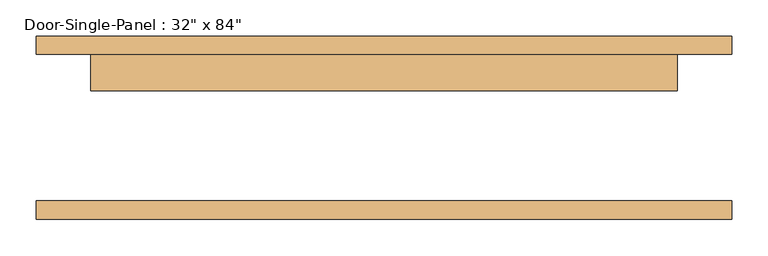
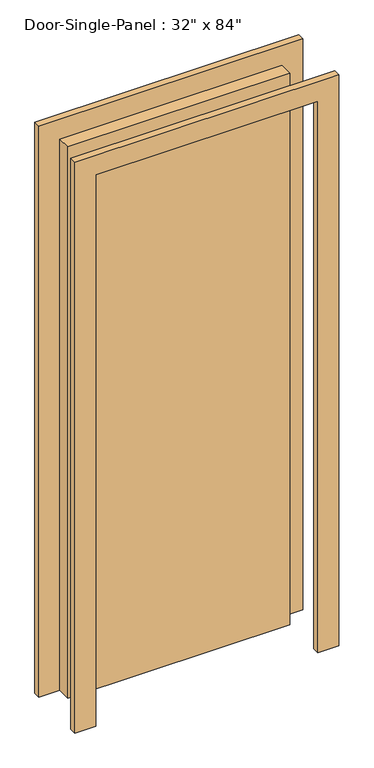
"""IFC4 building model written with IfcOpenShell, lengths in millimetres: door geometry."""

from ifc_helpers import new_model, si_unit, frame, origin, origin_with_axes, place, context, project, spatial, polyline, outline, extrude, source, transform, mapped, element, save


def door_70ddef25(model_context):
    return source(origin(), model_context, "Body", "SweptSolid", [
        extrude(outline(polyline([(406.4, 50.8), (-406.4, 50.8), (-406.4, 101.6), (406.4, 101.6), (406.4, 50.8)])), origin_with_axes(), (0.0, 0.0, 1.0), 2133.6),
        extrude(outline(polyline([(2209.8, -482.6), (0.0, -482.6), (0.0, -406.4), (2133.6, -406.4), (2133.6, 406.4), (0.0, 406.4), (0.0, 482.6), (2209.8, 482.6), (2209.8, -482.6)])), frame((0.0, 101.6, 0.0), z_axis=(0.0, 1.0, 0.0), x_axis=(0.0, 0.0, 1.0)), (0.0, 0.0, 1.0), 25.4),
        extrude(outline(polyline([(2209.8, 482.6), (2209.8, -482.6), (0.0, -482.6), (0.0, -406.4), (2133.6, -406.4), (2133.6, 406.4), (0.0, 406.4), (0.0, 482.6), (2209.8, 482.6)])), frame((0.0, -127.0, 0.0), z_axis=(0.0, 1.0, 0.0), x_axis=(0.0, 0.0, 1.0)), (0.0, 0.0, 1.0), 25.4),
    ])


if __name__ == "__main__":
    model = new_model("IFC4")
    model_context = context("Model", 3, world=origin())
    ifc_project = project(units=[si_unit("LENGTHUNIT", "METRE", prefix="MILLI")], contexts=[model_context])
    site = spatial("IfcSite", under=ifc_project)
    building = spatial("IfcBuilding", under=site)
    placement = place(None, origin())
    door_shape = door_70ddef25(model_context)
    element("IfcDoor", 1, ObjectType="Door-Single-Panel : 32\" x 84\"", at=placement, inside=building, context=model_context, shape_type="MappedRepresentation", body=[
        mapped(door_shape, transform((0.0, 0.0, 0.0), x_axis=(1.0, 0.0, 0.0), y_axis=(0.0, 1.0, 0.0), z_axis=(0.0, 0.0, 1.0))),
    ])
    save(model, "model.ifc")

# Revit data of these elements
# Type "Door-Single-Panel : 32\" x 84\""
#   Type Mark = "11"
#   Construction Type Id = "DOOR"
#   Assembly Code = "C1020300"
#   Analytic Construction = "Wooden"
#   Thickness = 0' - 2"
#   Thermal Resistance (R) = 2.5876 (h·ft²·°F)/BTU
#   Swing Angle [instance default] = 90.00°
#   Heat Transfer Coefficient (U) = 0.3865 BTU/(h·ft²·°F)
#   Height = 7' - 0"
#   Trim Projection Ext = 0' - 1"
#   Trim Projection Int = 0' - 1"
#   Trim Width = 0' - 3"
#   Width = 2' - 8"
#   Define Thermal Properties by = 1
#   Panel Material = Wood - Birch - Solid Stained Light Low Gloss
#   Trim Material = Paint - Sienna
#   Visual Light Transmittance = 0
#   Solar Heat Gain Coefficient = 0
#   Function = (empty or 0)
#   Wall Closure = (empty or 0)
# Element 1 (IfcDoor, "Door-Single-Panel : 32\" x 84\"")
#   Materials on its faces: "Paint - Sienna", "Wood - Birch - Solid Stained Light Low Gloss"
# Materials
#   "Wood - Birch - Solid Stained Light Low Gloss": class "Wood", colour RGB 210 159 95, transparency 0, Cost = 0
#   "Paint - Sienna": colour RGB 118 70 51, transparency 0, Cost = 0
